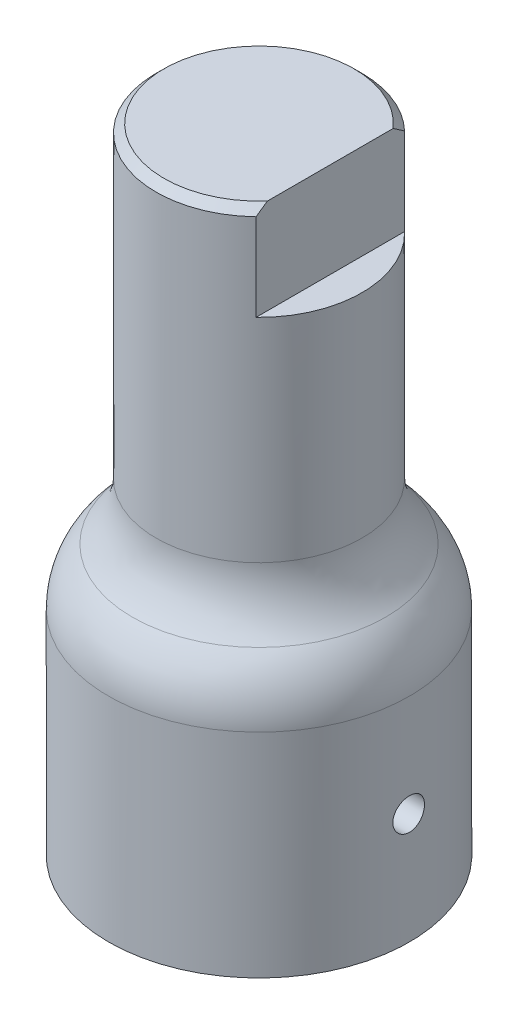
ISO-10303-21;
HEADER;
FILE_DESCRIPTION(('STEP AP214'),'2;1');
FILE_NAME('part.step','',(''),(''),'','','');
FILE_SCHEMA(('AUTOMOTIVE_DESIGN { 1 0 10303 214 1 1 1 1 }'));
ENDSEC;
DATA;
#1=APPLICATION_CONTEXT('core data for automotive mechanical design processes');
#2=APPLICATION_PROTOCOL_DEFINITION('international standard','automotive_design',2000,#1);
#3=PRODUCT_CONTEXT('',#1,'mechanical');
#4=PRODUCT('Part','Part','',(#3));
#5=PRODUCT_RELATED_PRODUCT_CATEGORY('part','',(#4));
#6=PRODUCT_DEFINITION_FORMATION('','',#4);
#7=PRODUCT_DEFINITION_CONTEXT('part definition',#1,'design');
#8=PRODUCT_DEFINITION('design','',#6,#7);
#9=PRODUCT_DEFINITION_SHAPE('','',#8);
#10=(LENGTH_UNIT() NAMED_UNIT(*) SI_UNIT(.MILLI.,.METRE.));
#11=(NAMED_UNIT(*) PLANE_ANGLE_UNIT() SI_UNIT($,.RADIAN.));
#12=(NAMED_UNIT(*) SI_UNIT($,.STERADIAN.) SOLID_ANGLE_UNIT());
#13=UNCERTAINTY_MEASURE_WITH_UNIT(LENGTH_MEASURE(1.E-05),#10,'distance_accuracy_value','');
#14=(GEOMETRIC_REPRESENTATION_CONTEXT(3) GLOBAL_UNCERTAINTY_ASSIGNED_CONTEXT((#13)) GLOBAL_UNIT_ASSIGNED_CONTEXT((#10,
#11,#12)) REPRESENTATION_CONTEXT('',''));
#15=CARTESIAN_POINT('',(0.,0.,0.));
#16=DIRECTION('',(0.,0.,1.));
#17=DIRECTION('',(1.,0.,0.));
#18=AXIS2_PLACEMENT_3D('',#15,#16,#17);
#19=CARTESIAN_POINT('',(0.,40.,0.));
#20=DIRECTION('',(0.,-1.,0.));
#21=DIRECTION('',(0.,0.,-1.));
#22=AXIS2_PLACEMENT_3D('',#19,#20,#21);
#23=CYLINDRICAL_SURFACE('',#22,6.5);
#24=CARTESIAN_POINT('',(0.,39.49999999999,0.));
#25=DIRECTION('',(0.,-1.,0.));
#26=DIRECTION('',(0.,0.,-1.));
#27=AXIS2_PLACEMENT_3D('',#24,#25,#26);
#28=CIRCLE('',#27,6.5);
#29=CARTESIAN_POINT('',(4.5,39.49999999999,-4.69041575982343));
#30=VERTEX_POINT('',#29);
#31=CARTESIAN_POINT('',(4.5,39.49999999999,4.69041575982343));
#32=VERTEX_POINT('',#31);
#33=EDGE_CURVE('E91',#30,#32,#28,.F.);
#34=ORIENTED_EDGE('',*,*,#33,.F.);
#35=DIRECTION('',(0.,1.,0.));
#36=VECTOR('',#35,1.);
#37=CARTESIAN_POINT('',(4.5,34.,-4.69041575982343));
#38=LINE('',#37,#36);
#39=CARTESIAN_POINT('',(4.5,34.,-4.69041575982343));
#40=VERTEX_POINT('',#39);
#41=EDGE_CURVE('E90',#40,#30,#38,.T.);
#42=ORIENTED_EDGE('',*,*,#41,.F.);
#43=CARTESIAN_POINT('',(0.,34.,0.));
#44=DIRECTION('',(0.,1.,0.));
#45=DIRECTION('',(0.,0.,1.));
#46=AXIS2_PLACEMENT_3D('',#43,#44,#45);
#47=CIRCLE('',#46,6.5);
#48=CARTESIAN_POINT('',(4.5,34.,4.69041575982343));
#49=VERTEX_POINT('',#48);
#50=EDGE_CURVE('E78',#49,#40,#47,.T.);
#51=ORIENTED_EDGE('',*,*,#50,.F.);
#52=DIRECTION('',(0.,1.,0.));
#53=VECTOR('',#52,1.);
#54=CARTESIAN_POINT('',(4.5,34.,4.69041575982343));
#55=LINE('',#54,#53);
#56=EDGE_CURVE('E86',#49,#32,#55,.T.);
#57=ORIENTED_EDGE('',*,*,#56,.T.);
#58=EDGE_LOOP('',(#34,#42,#51,#57));
#59=FACE_BOUND('',#58,.T.);
#60=CARTESIAN_POINT('',(0.,20.5825756949558,0.));
#61=DIRECTION('',(0.,-1.,0.));
#62=DIRECTION('',(0.,0.,-1.));
#63=AXIS2_PLACEMENT_3D('',#60,#61,#62);
#64=CIRCLE('',#63,6.5);
#65=CARTESIAN_POINT('',(0.,20.5825756949558,-6.5));
#66=VERTEX_POINT('',#65);
#67=EDGE_CURVE('E163',#66,#66,#64,.F.);
#68=ORIENTED_EDGE('',*,*,#67,.T.);
#69=EDGE_LOOP('',(#68));
#70=FACE_BOUND('',#69,.T.);
#71=ADVANCED_FACE('F37',(#59,#70),#23,.T.);
#72=CARTESIAN_POINT('',(0.,16.,0.));
#73=DIRECTION('',(0.,-1.,0.));
#74=DIRECTION('',(0.,0.,-1.));
#75=AXIS2_PLACEMENT_3D('',#72,#73,#74);
#76=CYLINDRICAL_SURFACE('',#75,9.5);
#77=CARTESIAN_POINT('',(9.44722181384559,7.,-1.));
#78=CARTESIAN_POINT('',(9.44722250266399,6.94399676022231,-0.999997582005042));
#79=CARTESIAN_POINT('',(9.44772516447025,6.8879568797022,-0.995279605314903));
#80=CARTESIAN_POINT('',(9.44968112934553,6.77743197119586,-0.976530575638432));
#81=CARTESIAN_POINT('',(9.45113546960823,6.72294870739155,-0.962489361408324));
#82=CARTESIAN_POINT('',(9.45482827329693,6.61715353672435,-0.925508243054439));
#83=CARTESIAN_POINT('',(9.45706625036201,6.56583968596353,-0.902573857494193));
#84=CARTESIAN_POINT('',(9.46207356819287,6.46780040586029,-0.848468268709648));
#85=CARTESIAN_POINT('',(9.46484280623326,6.42107409210137,-0.81729865742177));
#86=CARTESIAN_POINT('',(9.47061306994568,6.33333797951133,-0.747473131447723));
#87=CARTESIAN_POINT('',(9.47361488826576,6.29234919728408,-0.708790872156587));
#88=CARTESIAN_POINT('',(9.47950490283494,6.21743276042639,-0.625094500148442));
#89=CARTESIAN_POINT('',(9.4823930937953,6.18350543415458,-0.580080093148769));
#90=CARTESIAN_POINT('',(9.48773832873555,6.12360171385311,-0.484867702730017));
#91=CARTESIAN_POINT('',(9.49019435323658,6.09764401557964,-0.434657894607719));
#92=CARTESIAN_POINT('',(9.49438988246007,6.05453602526003,-0.330561942132097));
#93=CARTESIAN_POINT('',(9.49612940639459,6.03738549705754,-0.276675896397674));
#94=CARTESIAN_POINT('',(9.49869036912673,6.01244058881074,-0.166970075945796));
#95=CARTESIAN_POINT('',(9.4995152042548,6.00461158896824,-0.111158253620166));
#96=CARTESIAN_POINT('',(9.50016541360392,5.99842482083021,0.000992835185780201));
#97=CARTESIAN_POINT('',(9.49999081632174,6.00006678248953,0.0573320865818019));
#98=CARTESIAN_POINT('',(9.49866460674142,6.01274729442015,0.168703652078324));
#99=CARTESIAN_POINT('',(9.4975168652733,6.02374861698648,0.223740257380179));
#100=CARTESIAN_POINT('',(9.49437776823862,6.05477752943278,0.331181565951237));
#101=CARTESIAN_POINT('',(9.49238640070667,6.07480524733706,0.38358623187907));
#102=CARTESIAN_POINT('',(9.48777724512953,6.12335901820799,0.484393029454015));
#103=CARTESIAN_POINT('',(9.4851582498829,6.15190147495144,0.532787202758796));
#104=CARTESIAN_POINT('',(9.47958754859329,6.21666259333303,0.624112447479543));
#105=CARTESIAN_POINT('',(9.47663583173319,6.25288150457432,0.667043341182004));
#106=CARTESIAN_POINT('',(9.47071386481717,6.33217661549575,0.746441553980417));
#107=CARTESIAN_POINT('',(9.46774359429256,6.37528521174329,0.782876524755556));
#108=CARTESIAN_POINT('',(9.46213353822369,6.467023875572,0.847998010788903));
#109=CARTESIAN_POINT('',(9.45949375324791,6.51565395265044,0.876684512719002));
#110=CARTESIAN_POINT('',(9.45484337668269,6.61708076887816,0.925494983579704));
#111=CARTESIAN_POINT('',(9.45283294031977,6.66987853195736,0.945616840511516));
#112=CARTESIAN_POINT('',(9.44967206522172,6.77812918602637,0.976700646432597));
#113=CARTESIAN_POINT('',(9.44852159738819,6.83358198711122,0.987662905352753));
#114=CARTESIAN_POINT('',(9.44721601825639,6.94528430332103,1.00007449042647));
#115=CARTESIAN_POINT('',(9.44705616649923,7.0015287310886,1.00156912338335));
#116=CARTESIAN_POINT('',(9.44773740410882,7.11346722487839,0.995122122181052));
#117=CARTESIAN_POINT('',(9.44857847846089,7.16916129914371,0.98718062957116));
#118=CARTESIAN_POINT('',(9.45116248557082,7.27828536167683,0.962124760080199));
#119=CARTESIAN_POINT('',(9.45290330202064,7.33172034594203,0.945031905000058));
#120=CARTESIAN_POINT('',(9.457088931172,7.43496489295997,0.902180520375011));
#121=CARTESIAN_POINT('',(9.45953376168103,7.48477436396822,0.876421771630251));
#122=CARTESIAN_POINT('',(9.46486340159122,7.57956019358576,0.816856703395602));
#123=CARTESIAN_POINT('',(9.46774983441864,7.6245176301711,0.783020420843189));
#124=CARTESIAN_POINT('',(9.47363218095351,7.70813110460675,0.708303604881553));
#125=CARTESIAN_POINT('',(9.47662809766472,7.74678696941029,0.667422878089));
#126=CARTESIAN_POINT('',(9.48240620792166,7.81685680342479,0.579580811033078));
#127=CARTESIAN_POINT('',(9.48518749827024,7.84824117481112,0.532595793455961));
#128=CARTESIAN_POINT('',(9.49020976547322,7.90267324792291,0.433995477074838));
#129=CARTESIAN_POINT('',(9.49245075042118,7.92572107452906,0.38238024764545));
#130=CARTESIAN_POINT('',(9.49613584419318,7.96277590812539,0.276087032602508));
#131=CARTESIAN_POINT('',(9.49758151475308,7.97680064274985,0.221415283364815));
#132=CARTESIAN_POINT('',(9.49951951574434,7.99546900480972,0.11047692402959));
#133=CARTESIAN_POINT('',(9.50001187606999,8.00011292641273,0.0542103639989369));
#134=CARTESIAN_POINT('',(9.49998774184331,7.9998834442607,-0.0580300347921259));
#135=CARTESIAN_POINT('',(9.49947611139555,7.99505592746934,-0.11400397405403));
#136=CARTESIAN_POINT('',(9.49751109070018,7.97611701178647,-0.224340884848705));
#137=CARTESIAN_POINT('',(9.49605769994164,7.96200560785844,-0.278703855507504));
#138=CARTESIAN_POINT('',(9.49237193768829,7.92491254193537,-0.384274195424411));
#139=CARTESIAN_POINT('',(9.490139699013,7.90193239228629,-0.435482100975531));
#140=CARTESIAN_POINT('',(9.48514475079928,7.84775899475027,-0.53332131052237));
#141=CARTESIAN_POINT('',(9.48238204252499,7.81656576643549,-0.579952625423968));
#142=CARTESIAN_POINT('',(9.4766194383916,7.74667994304738,-0.667550047988318));
#143=CARTESIAN_POINT('',(9.47361849971248,7.70795316285625,-0.708488814694208));
#144=CARTESIAN_POINT('',(9.46772640505434,7.62416800248141,-0.783306479853839));
#145=CARTESIAN_POINT('',(9.46483527551713,7.57910810942172,-0.817183686602055));
#146=CARTESIAN_POINT('',(9.45948152841544,7.48379663846925,-0.876992670192276));
#147=CARTESIAN_POINT('',(9.4570201280027,7.43353093654307,-0.902902032073807));
#148=CARTESIAN_POINT('',(9.45281896154563,7.3293677382227,-0.945877463600506));
#149=CARTESIAN_POINT('',(9.45107838754954,7.2754743871793,-0.962953439690975));
#150=CARTESIAN_POINT('',(9.44895178678448,7.18440056938451,-0.983551575010372));
#151=CARTESIAN_POINT('',(9.44830614572659,7.14780098379419,-0.989711221415895));
#152=CARTESIAN_POINT('',(9.44744093225495,7.07413961758953,-0.997936224550727));
#153=CARTESIAN_POINT('',(9.44722135780237,7.03707783918775,-1.00000160087218));
#154=CARTESIAN_POINT('',(9.44722181384559,7.,-1.));
#155=B_SPLINE_CURVE_WITH_KNOTS('',3,(#77,#78,#79,#80,#81,#82,#83,#84,#85,#86,#87,#88,#89,#90,
#91,#92,#93,#94,#95,#96,#97,#98,#99,#100,#101,#102,#103,#104,#105,#106,#107,#108,#109,#110,#111,
#112,#113,#114,#115,#116,#117,#118,#119,#120,#121,#122,#123,#124,#125,#126,#127,#128,#129,#130,
#131,#132,#133,#134,#135,#136,#137,#138,#139,#140,#141,#142,#143,#144,#145,#146,#147,#148,#149,
#150,#151,#152,#153,#154),.UNSPECIFIED.,.T.,.F.,(4,2,2,2,2,2,2,2,2,2,2,2,2,2,2,2,2,2,2,2,2,2,2,
2,2,2,2,2,2,2,2,2,2,2,2,2,2,2,4),(0.,0.167874308515836,0.335931881467919,0.503885334527946,
0.671806344537529,0.840327196784644,1.00885588352368,1.17777694897953,1.34669348473242,
1.51498069435804,1.68326310564076,1.8508792712072,2.01849781420309,2.18644138555292,
2.35439041849688,2.52315376360364,2.69191739899767,2.86072262658684,3.02952214212699,
3.19751326274829,3.36550186340294,3.53309711962096,3.70069661540383,3.86892774419037,
4.03716349197577,4.20607244449903,4.37497886667638,4.54355241740059,4.71212068184014,
4.87987428784667,5.04762798486011,5.21535308824674,5.38307779193977,5.55158212557546,
5.72012678074431,5.8891413337759,6.05796592756899,6.16911032609435,6.28025419276375),.UNSPECIFIED.);
#156=CARTESIAN_POINT('',(9.44722181384559,7.,-1.));
#157=VERTEX_POINT('',#156);
#158=EDGE_CURVE('E88',#157,#157,#155,.T.);
#159=ORIENTED_EDGE('',*,*,#158,.T.);
#160=EDGE_LOOP('',(#159));
#161=FACE_BOUND('',#160,.T.);
#162=CARTESIAN_POINT('',(0.,13.441147266413,0.));
#163=DIRECTION('',(0.,-1.,0.));
#164=DIRECTION('',(0.,0.,-1.));
#165=AXIS2_PLACEMENT_3D('',#162,#163,#164);
#166=CIRCLE('',#165,9.5);
#167=CARTESIAN_POINT('',(0.,13.441147266413,-9.5));
#168=VERTEX_POINT('',#167);
#169=EDGE_CURVE('E53',#168,#168,#166,.T.);
#170=ORIENTED_EDGE('',*,*,#169,.T.);
#171=EDGE_LOOP('',(#170));
#172=FACE_BOUND('',#171,.T.);
#173=CARTESIAN_POINT('',(0.,0.,0.));
#174=DIRECTION('',(0.,1.,0.));
#175=DIRECTION('',(0.,0.,1.));
#176=AXIS2_PLACEMENT_3D('',#173,#174,#175);
#177=CIRCLE('',#176,9.5);
#178=CARTESIAN_POINT('',(0.,0.,9.5));
#179=VERTEX_POINT('',#178);
#180=EDGE_CURVE('E160',#179,#179,#177,.T.);
#181=ORIENTED_EDGE('',*,*,#180,.T.);
#182=EDGE_LOOP('',(#181));
#183=FACE_BOUND('',#182,.T.);
#184=ADVANCED_FACE('F128',(#161,#172,#183),#76,.T.);
#185=CARTESIAN_POINT('',(0.,0.,0.));
#186=DIRECTION('',(0.,1.,0.));
#187=DIRECTION('',(0.,0.,1.));
#188=AXIS2_PLACEMENT_3D('',#185,#186,#187);
#189=PLANE('',#188);
#190=CARTESIAN_POINT('',(0.,0.,0.));
#191=DIRECTION('',(0.,-1.,0.));
#192=DIRECTION('',(0.,0.,-1.));
#193=AXIS2_PLACEMENT_3D('',#190,#191,#192);
#194=CIRCLE('',#193,6.);
#195=CARTESIAN_POINT('',(0.,0.,-6.));
#196=VERTEX_POINT('',#195);
#197=EDGE_CURVE('E221',#196,#196,#194,.T.);
#198=ORIENTED_EDGE('',*,*,#197,.F.);
#199=EDGE_LOOP('',(#198));
#200=FACE_BOUND('',#199,.T.);
#201=ORIENTED_EDGE('',*,*,#180,.F.);
#202=EDGE_LOOP('',(#201));
#203=FACE_BOUND('',#202,.T.);
#204=ADVANCED_FACE('F135',(#200,#203),#189,.F.);
#205=CARTESIAN_POINT('',(0.,20.5825756949558,0.));
#206=DIRECTION('',(0.,-1.,0.));
#207=DIRECTION('',(0.,0.,-1.));
#208=AXIS2_PLACEMENT_3D('',#205,#206,#207);
#209=TOROIDAL_SURFACE('',#208,11.5,5.);
#210=CARTESIAN_POINT('',(0.,17.0118614806844,0.));
#211=DIRECTION('',(0.,1.,0.));
#212=DIRECTION('',(0.,0.,1.));
#213=AXIS2_PLACEMENT_3D('',#210,#211,#212);
#214=CIRCLE('',#213,8.);
#215=CARTESIAN_POINT('',(0.,17.0118614806844,8.));
#216=VERTEX_POINT('',#215);
#217=EDGE_CURVE('E168',#216,#216,#214,.T.);
#218=ORIENTED_EDGE('',*,*,#217,.T.);
#219=EDGE_LOOP('',(#218));
#220=FACE_BOUND('',#219,.T.);
#221=ORIENTED_EDGE('',*,*,#67,.F.);
#222=EDGE_LOOP('',(#221));
#223=FACE_BOUND('',#222,.T.);
#224=ADVANCED_FACE('F139',(#220,#223),#209,.F.);
#225=CARTESIAN_POINT('',(0.,13.441147266413,0.));
#226=DIRECTION('',(0.,-1.,0.));
#227=DIRECTION('',(0.,0.,-1.));
#228=AXIS2_PLACEMENT_3D('',#225,#226,#227);
#229=DEGENERATE_TOROIDAL_SURFACE('',#228,4.5,5.,.T.);
#230=ORIENTED_EDGE('',*,*,#169,.F.);
#231=EDGE_LOOP('',(#230));
#232=FACE_BOUND('',#231,.T.);
#233=ORIENTED_EDGE('',*,*,#217,.F.);
#234=EDGE_LOOP('',(#233));
#235=FACE_BOUND('',#234,.T.);
#236=ADVANCED_FACE('F45',(#232,#235),#229,.T.);
#237=CARTESIAN_POINT('',(0.,40.,0.));
#238=DIRECTION('',(0.,-1.,0.));
#239=DIRECTION('',(0.,0.,1.));
#240=AXIS2_PLACEMENT_3D('',#237,#238,#239);
#241=CONICAL_SURFACE('',#240,6.,0.785398163387451);
#242=CARTESIAN_POINT('',(4.5,39.4994948602286,-4.69111575982343));
#243=CARTESIAN_POINT('',(4.5,39.5910625718077,-4.56419132998681));
#244=CARTESIAN_POINT('',(4.5,39.6815022347654,-4.43643607105073));
#245=CARTESIAN_POINT('',(4.5,39.8595893158656,-4.17892229941567));
#246=CARTESIAN_POINT('',(4.5,39.9472356185483,-4.04916301641921));
#247=CARTESIAN_POINT('',(4.5,40.1201204357677,-3.78588595282148));
#248=CARTESIAN_POINT('',(4.5,40.2053193928018,-3.65234206231063));
#249=CARTESIAN_POINT('',(4.5,40.3714251731154,-3.38262522364676));
#250=CARTESIAN_POINT('',(4.5,40.4523324373673,-3.2464525475707));
#251=CARTESIAN_POINT('',(4.5,40.6119674205422,-2.96559683200244));
#252=CARTESIAN_POINT('',(4.5,40.6904812028258,-2.82079052248245));
#253=CARTESIAN_POINT('',(4.5,40.8403076188372,-2.52751600449652));
#254=CARTESIAN_POINT('',(4.5,40.9116188551767,-2.37904709236322));
#255=CARTESIAN_POINT('',(4.5,41.1114016258523,-1.92884045725228));
#256=CARTESIAN_POINT('',(4.5,41.2266603751218,-1.62072923163736));
#257=CARTESIAN_POINT('',(4.5,41.3559192389052,-1.15662252410079));
#258=CARTESIAN_POINT('',(4.5,41.3912152564831,-1.00651231509382));
#259=CARTESIAN_POINT('',(4.5,41.4477583690889,-0.703576641579641));
#260=CARTESIAN_POINT('',(4.5,41.4690035145624,-0.550750803299149));
#261=CARTESIAN_POINT('',(4.5,41.4957872742846,-0.246125362524782));
#262=CARTESIAN_POINT('',(4.5,41.501567030541,-0.0943472645680615));
#263=CARTESIAN_POINT('',(4.5,41.4977026039483,0.20900812846482));
#264=CARTESIAN_POINT('',(4.5,41.488058668143,0.360585426718301));
#265=CARTESIAN_POINT('',(4.5,41.4541105883571,0.661323608614883));
#266=CARTESIAN_POINT('',(4.5,41.42987648739,0.810492562778165));
#267=CARTESIAN_POINT('',(4.5,41.3683165849852,1.1060800923311));
#268=CARTESIAN_POINT('',(4.5,41.3309887502376,1.25249823682824));
#269=CARTESIAN_POINT('',(4.5,41.2445112690977,1.54414346716479));
#270=CARTESIAN_POINT('',(4.5,41.1951928475382,1.689319822961));
#271=CARTESIAN_POINT('',(4.5,41.0870489717548,1.97603473847701));
#272=CARTESIAN_POINT('',(4.5,41.0282237295574,2.1175733792456));
#273=CARTESIAN_POINT('',(4.5,40.866702735929,2.47783478069375));
#274=CARTESIAN_POINT('',(4.5,40.758276270693,2.6939778478982));
#275=CARTESIAN_POINT('',(4.5,40.5277107571137,3.11894516522701));
#276=CARTESIAN_POINT('',(4.5,40.4055578240113,3.3277617191103));
#277=CARTESIAN_POINT('',(4.5,40.1560956473342,3.73168648275101));
#278=CARTESIAN_POINT('',(4.5,40.0291424867711,3.92701626465144));
#279=CARTESIAN_POINT('',(4.5,39.8337936410973,4.21629165571739));
#280=CARTESIAN_POINT('',(4.5,39.7679449930584,4.31197670619119));
#281=CARTESIAN_POINT('',(4.5,39.6347749295762,4.50229951775167));
#282=CARTESIAN_POINT('',(4.5,39.5674536972453,4.59693740687134));
#283=CARTESIAN_POINT('',(4.5,39.4994948602286,4.69111575982343));
#284=B_SPLINE_CURVE_WITH_KNOTS('',3,(#242,#243,#244,#245,#246,#247,#248,#249,#250,#251,#252,
#253,#254,#255,#256,#257,#258,#259,#260,#261,#262,#263,#264,#265,#266,#267,#268,#269,#270,#271,
#272,#273,#274,#275,#276,#277,#278,#279,#280,#281,#282,#283),.UNSPECIFIED.,.F.,.F.,(4,2,2,2,2,2,
2,2,2,2,2,2,2,2,2,2,2,2,2,2,4),(0.,0.469535108464433,0.939255422972653,1.41440686748524,
1.88950939514254,2.38346750420522,2.87752126427259,3.86015474528862,4.32222813434726,
4.78436562250868,5.23925412221588,5.69413533597521,6.14685002273307,6.59963504214774,
7.05920535362152,7.51876541691527,8.24345222400739,8.96887878807251,9.66756320143564,
10.0160138353499,10.3644213838166),.UNSPECIFIED.);
#285=CARTESIAN_POINT('',(4.5,40.,-3.96862696659689));
#286=VERTEX_POINT('',#285);
#287=EDGE_CURVE('E62',#30,#286,#284,.T.);
#288=ORIENTED_EDGE('',*,*,#287,.F.);
#289=ORIENTED_EDGE('',*,*,#33,.T.);
#290=CARTESIAN_POINT('',(4.5,40.,3.96862696659689));
#291=VERTEX_POINT('',#290);
#292=EDGE_CURVE('E69',#291,#32,#284,.T.);
#293=ORIENTED_EDGE('',*,*,#292,.F.);
#294=CARTESIAN_POINT('',(0.,40.,0.));
#295=DIRECTION('',(0.,1.,0.));
#296=DIRECTION('',(0.,0.,1.));
#297=AXIS2_PLACEMENT_3D('',#294,#295,#296);
#298=CIRCLE('',#297,6.);
#299=EDGE_CURVE('E106',#286,#291,#298,.T.);
#300=ORIENTED_EDGE('',*,*,#299,.F.);
#301=EDGE_LOOP('',(#288,#289,#293,#300));
#302=FACE_BOUND('',#301,.T.);
#303=ADVANCED_FACE('F108',(#302),#241,.T.);
#304=CARTESIAN_POINT('',(0.,40.,0.));
#305=DIRECTION('',(0.,1.,0.));
#306=DIRECTION('',(0.,0.,1.));
#307=AXIS2_PLACEMENT_3D('',#304,#305,#306);
#308=PLANE('',#307);
#309=DIRECTION('',(0.,0.,1.));
#310=VECTOR('',#309,1.);
#311=CARTESIAN_POINT('',(4.5,40.,0.));
#312=LINE('',#311,#310);
#313=EDGE_CURVE('E12',#286,#291,#312,.T.);
#314=ORIENTED_EDGE('',*,*,#313,.F.);
#315=ORIENTED_EDGE('',*,*,#299,.T.);
#316=EDGE_LOOP('',(#314,#315));
#317=FACE_BOUND('',#316,.T.);
#318=ADVANCED_FACE('F112',(#317),#308,.T.);
#319=CARTESIAN_POINT('',(4.5,34.,-4.69041575982343));
#320=DIRECTION('',(-1.,0.,0.));
#321=DIRECTION('',(0.,0.,1.));
#322=AXIS2_PLACEMENT_3D('',#319,#320,#321);
#323=PLANE('',#322);
#324=ORIENTED_EDGE('',*,*,#287,.T.);
#325=ORIENTED_EDGE('',*,*,#313,.T.);
#326=ORIENTED_EDGE('',*,*,#292,.T.);
#327=ORIENTED_EDGE('',*,*,#56,.F.);
#328=DIRECTION('',(0.,0.,1.));
#329=VECTOR('',#328,1.);
#330=CARTESIAN_POINT('',(4.5,34.,-4.69041575982343));
#331=LINE('',#330,#329);
#332=EDGE_CURVE('E84',#40,#49,#331,.T.);
#333=ORIENTED_EDGE('',*,*,#332,.F.);
#334=ORIENTED_EDGE('',*,*,#41,.T.);
#335=EDGE_LOOP('',(#324,#325,#326,#327,#333,#334));
#336=FACE_BOUND('',#335,.T.);
#337=ADVANCED_FACE('F87',(#336),#323,.F.);
#338=CARTESIAN_POINT('',(0.,34.,0.));
#339=DIRECTION('',(0.,1.,0.));
#340=DIRECTION('',(0.,0.,1.));
#341=AXIS2_PLACEMENT_3D('',#338,#339,#340);
#342=PLANE('',#341);
#343=ORIENTED_EDGE('',*,*,#50,.T.);
#344=ORIENTED_EDGE('',*,*,#332,.T.);
#345=EDGE_LOOP('',(#343,#344));
#346=FACE_BOUND('',#345,.T.);
#347=ADVANCED_FACE('F85',(#346),#342,.T.);
#348=CARTESIAN_POINT('',(-3.5,7.,0.));
#349=DIRECTION('',(1.,0.,0.));
#350=DIRECTION('',(0.,0.,-1.));
#351=AXIS2_PLACEMENT_3D('',#348,#349,#350);
#352=CYLINDRICAL_SURFACE('',#351,1.);
#353=CARTESIAN_POINT('',(5.91607978309962,7.,-1.));
#354=CARTESIAN_POINT('',(5.91608078960511,6.94424970074159,-0.999997759368403));
#355=CARTESIAN_POINT('',(5.91687637019227,6.88846895759005,-0.99532206761493));
#356=CARTESIAN_POINT('',(5.91996982947271,6.77847258271193,-0.976750971230158));
#357=CARTESIAN_POINT('',(5.92226909356571,6.72425844250019,-0.962847064123862));
#358=CARTESIAN_POINT('',(5.9281024372893,6.61900308665729,-0.926251817466858));
#359=CARTESIAN_POINT('',(5.9316354846878,6.56795926053347,-0.903567821972436));
#360=CARTESIAN_POINT('',(5.93953708845736,6.47040761811452,-0.850074598756148));
#361=CARTESIAN_POINT('',(5.94390555078989,6.4238992921695,-0.819266285400629));
#362=CARTESIAN_POINT('',(5.95303388461044,6.33627486010173,-0.750075010786521));
#363=CARTESIAN_POINT('',(5.95779686930827,6.29520994744539,-0.71162761957291));
#364=CARTESIAN_POINT('',(5.96714992267783,6.22008267725539,-0.628388801878137));
#365=CARTESIAN_POINT('',(5.97173998108788,6.18602073475386,-0.583596999659996));
#366=CARTESIAN_POINT('',(5.98026294792988,6.12567417311226,-0.488609147979336));
#367=CARTESIAN_POINT('',(5.98419176972911,6.09943719690727,-0.438382432582682));
#368=CARTESIAN_POINT('',(5.99091494782862,6.05579157178779,-0.33415824868955));
#369=CARTESIAN_POINT('',(5.9937093778907,6.03838234884605,-0.280161025631277));
#370=CARTESIAN_POINT('',(5.99782693889752,6.01304298600644,-0.170457490537698));
#371=CARTESIAN_POINT('',(5.99916341244362,6.00502683359812,-0.11477155467171));
#372=CARTESIAN_POINT('',(6.00026031737113,5.99843369833896,-0.00283011421032022));
#373=CARTESIAN_POINT('',(6.00002085587723,5.99985607390111,0.0534253514115582));
#374=CARTESIAN_POINT('',(5.99800343372556,6.01203254061128,0.164320874031549));
#375=CARTESIAN_POINT('',(5.99624073476959,6.02269406536366,0.218971412280056));
#376=CARTESIAN_POINT('',(5.99139191508655,6.0529004296986,0.325696791844716));
#377=CARTESIAN_POINT('',(5.98830575405285,6.0724455398358,0.377771554660601));
#378=CARTESIAN_POINT('',(5.98113079404783,6.11995625612613,0.478142459113058));
#379=CARTESIAN_POINT('',(5.97703746930752,6.14796000483298,0.526420209207617));
#380=CARTESIAN_POINT('',(5.96830295228599,6.21156512905402,0.617626211938656));
#381=CARTESIAN_POINT('',(5.96366171567654,6.24716711948433,0.66055403116635));
#382=CARTESIAN_POINT('',(5.95428107293039,6.32547152264772,0.740388509378666));
#383=CARTESIAN_POINT('',(5.94954115892417,6.36825483796039,0.777215800901282));
#384=CARTESIAN_POINT('',(5.94055183913922,6.45943483608633,0.843181835379225));
#385=CARTESIAN_POINT('',(5.9363024378853,6.50783157067313,0.872320507412966));
#386=CARTESIAN_POINT('',(5.92877501824727,6.60895665675099,0.922097773795314));
#387=CARTESIAN_POINT('',(5.92549809321041,6.66168979923684,0.942726810911696));
#388=CARTESIAN_POINT('',(5.92030475475952,6.76993962892302,0.974811948326246));
#389=CARTESIAN_POINT('',(5.91838822155329,6.82545607057297,0.986268856307181));
#390=CARTESIAN_POINT('',(5.91615583768847,6.93698646246485,0.999572753951706));
#391=CARTESIAN_POINT('',(5.91582114303468,6.99298655188084,1.00153288316498));
#392=CARTESIAN_POINT('',(5.91674013912945,7.10451466867633,0.996089081072982));
#393=CARTESIAN_POINT('',(5.91799376852741,7.16004271420559,0.988685511449865));
#394=CARTESIAN_POINT('',(5.92193074982007,7.26869110367634,0.964820933971238));
#395=CARTESIAN_POINT('',(5.92460500767339,7.3218244559512,0.948417516258553));
#396=CARTESIAN_POINT('',(5.93107429202201,7.42458806651179,0.90707927607691));
#397=CARTESIAN_POINT('',(5.93486938556232,7.47421811502036,0.882143943240373));
#398=CARTESIAN_POINT('',(5.94319651358957,7.56906983776245,0.824182669291689));
#399=CARTESIAN_POINT('',(5.94773502240139,7.61424662910242,0.791084225663744));
#400=CARTESIAN_POINT('',(5.95701866671947,7.698445413078,0.717835786283191));
#401=CARTESIAN_POINT('',(5.96176381674132,7.7374669724439,0.677685294553617));
#402=CARTESIAN_POINT('',(5.97098568847306,7.80866075709148,0.590971228131523));
#403=CARTESIAN_POINT('',(5.97545910537869,7.84075753051382,0.544345301354478));
#404=CARTESIAN_POINT('',(5.98358044973177,7.89666213080195,0.44629737917973));
#405=CARTESIAN_POINT('',(5.9872284038799,7.92047022578954,0.39487553898825));
#406=CARTESIAN_POINT('',(5.99327343267833,7.95900423358195,0.28891962060053));
#407=CARTESIAN_POINT('',(5.99567593827049,7.97376963029397,0.234400225041043));
#408=CARTESIAN_POINT('',(5.99898233267713,7.99392623958553,0.123612293949684));
#409=CARTESIAN_POINT('',(5.99988634480071,7.99931822349294,0.0673439027286485));
#410=CARTESIAN_POINT('',(6.0000921515513,8.00055275292488,-0.0446165103094735));
#411=CARTESIAN_POINT('',(5.99941320809696,7.99651010157642,-0.100307264241073));
#412=CARTESIAN_POINT('',(5.99656871354913,7.97923843109224,-0.210204789725878));
#413=CARTESIAN_POINT('',(5.99440317078001,7.96600946339618,-0.264411569586971));
#414=CARTESIAN_POINT('',(5.98882795531034,7.9307847337825,-0.369758578367438));
#415=CARTESIAN_POINT('',(5.98541966816622,7.90879873271582,-0.42090214886161));
#416=CARTESIAN_POINT('',(5.97773102750941,7.85669682550793,-0.518792181192787));
#417=CARTESIAN_POINT('',(5.97345063265953,7.82658053397561,-0.565538434446987));
#418=CARTESIAN_POINT('',(5.96443051847589,7.7586659630152,-0.653885178210865));
#419=CARTESIAN_POINT('',(5.95968609820294,7.72078361809725,-0.695420572242247));
#420=CARTESIAN_POINT('',(5.95030521321901,7.63858867684072,-0.771585550379218));
#421=CARTESIAN_POINT('',(5.94566877405441,7.59427457644338,-0.806213514680477));
#422=CARTESIAN_POINT('',(5.93699337428039,7.50010187099694,-0.867805708367846));
#423=CARTESIAN_POINT('',(5.93295887192494,7.45020626406478,-0.894713995637817));
#424=CARTESIAN_POINT('',(5.92599684088708,7.34655630563543,-0.939725814576366));
#425=CARTESIAN_POINT('',(5.92306820700509,7.29280587092124,-0.957838142092642));
#426=CARTESIAN_POINT('',(5.91929897935112,7.19903849220933,-0.980810421248859));
#427=CARTESIAN_POINT('',(5.91809849368407,7.15958927681662,-0.987994967068113));
#428=CARTESIAN_POINT('',(5.91648854114608,7.08009860606356,-0.99759051807297));
#429=CARTESIAN_POINT('',(5.91607905991511,7.04005716146793,-1.00000160991677));
#430=CARTESIAN_POINT('',(5.91607978309962,7.,-1.));
#431=B_SPLINE_CURVE_WITH_KNOTS('',3,(#353,#354,#355,#356,#357,#358,#359,#360,#361,#362,#363,
#364,#365,#366,#367,#368,#369,#370,#371,#372,#373,#374,#375,#376,#377,#378,#379,#380,#381,#382,
#383,#384,#385,#386,#387,#388,#389,#390,#391,#392,#393,#394,#395,#396,#397,#398,#399,#400,#401,
#402,#403,#404,#405,#406,#407,#408,#409,#410,#411,#412,#413,#414,#415,#416,#417,#418,#419,#420,
#421,#422,#423,#424,#425,#426,#427,#428,#429,#430),.UNSPECIFIED.,.T.,.F.,(4,2,2,2,2,2,2,2,2,2,2,
2,2,2,2,2,2,2,2,2,2,2,2,2,2,2,2,2,2,2,2,2,2,2,2,2,2,2,4),(0.,0.167104415562128,0.33436300796778,
0.501481999132667,0.668582189603687,0.83715663660545,1.00574107132038,1.17533192042833,
1.34491174042704,1.51292626987285,1.68092937859336,1.84726848464127,2.01361265698072,
2.18071841654029,2.34783770488965,2.51698449383108,2.68613284296667,2.85547064997701,
3.0247935437349,3.19209416966423,3.3593883336385,3.52562425852456,3.69187012915689,
3.8596493710334,4.02744041770535,4.19697645212412,4.36650700188939,4.53529193765318,
4.704062983632,4.87079110504626,5.03751829285789,5.20406015931242,5.37060992155193,
5.5390679898356,5.70756551550984,5.8772549104514,6.04677426695051,6.16684268214775,
6.28690891757997),.UNSPECIFIED.);
#432=CARTESIAN_POINT('',(5.91607978309962,7.,-1.));
#433=VERTEX_POINT('',#432);
#434=EDGE_CURVE('E42',#433,#433,#431,.T.);
#435=ORIENTED_EDGE('',*,*,#434,.T.);
#436=EDGE_LOOP('',(#435));
#437=FACE_BOUND('',#436,.T.);
#438=ORIENTED_EDGE('',*,*,#158,.F.);
#439=EDGE_LOOP('',(#438));
#440=FACE_BOUND('',#439,.T.);
#441=ADVANCED_FACE('F116',(#437,#440),#352,.F.);
#442=CARTESIAN_POINT('',(0.,14.,0.));
#443=DIRECTION('',(0.,-1.,0.));
#444=DIRECTION('',(0.,0.,-1.));
#445=AXIS2_PLACEMENT_3D('',#442,#443,#444);
#446=CYLINDRICAL_SURFACE('',#445,6.);
#447=ORIENTED_EDGE('',*,*,#197,.T.);
#448=EDGE_LOOP('',(#447));
#449=FACE_BOUND('',#448,.T.);
#450=CARTESIAN_POINT('',(0.,14.,0.));
#451=DIRECTION('',(0.,-1.,0.));
#452=DIRECTION('',(0.,0.,-1.));
#453=AXIS2_PLACEMENT_3D('',#450,#451,#452);
#454=CIRCLE('',#453,6.);
#455=CARTESIAN_POINT('',(0.,14.,-6.));
#456=VERTEX_POINT('',#455);
#457=EDGE_CURVE('E222',#456,#456,#454,.T.);
#458=ORIENTED_EDGE('',*,*,#457,.F.);
#459=EDGE_LOOP('',(#458));
#460=FACE_BOUND('',#459,.T.);
#461=ORIENTED_EDGE('',*,*,#434,.F.);
#462=EDGE_LOOP('',(#461));
#463=FACE_BOUND('',#462,.T.);
#464=ADVANCED_FACE('F118',(#449,#460,#463),#446,.F.);
#465=CARTESIAN_POINT('',(0.,14.,0.));
#466=DIRECTION('',(0.,-1.,0.));
#467=DIRECTION('',(0.,0.,-1.));
#468=AXIS2_PLACEMENT_3D('',#465,#466,#467);
#469=PLANE('',#468);
#470=ORIENTED_EDGE('',*,*,#457,.T.);
#471=EDGE_LOOP('',(#470));
#472=FACE_BOUND('',#471,.T.);
#473=ADVANCED_FACE('F208',(#472),#469,.T.);
#474=CLOSED_SHELL('',(#71,#184,#204,#224,#236,#303,#318,#337,#347,#441,#464,#473));
#475=MANIFOLD_SOLID_BREP('B2',#474);
#476=ADVANCED_BREP_SHAPE_REPRESENTATION('',(#18,#475),#14);
#477=SHAPE_DEFINITION_REPRESENTATION(#9,#476);
ENDSEC;
END-ISO-10303-21;
